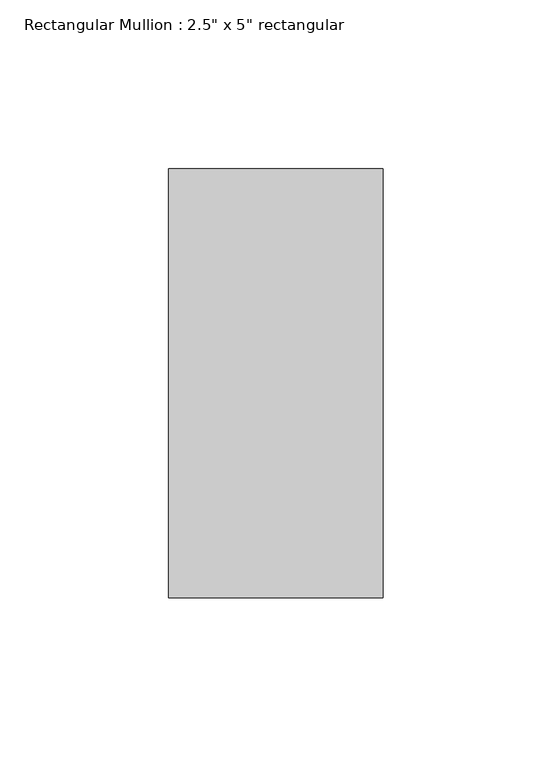
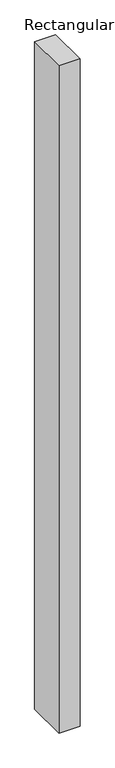
"""IFC4 building model written with IfcOpenShell, lengths in millimetres: member geometry."""

from ifc_helpers import new_model, si_unit, frame, origin, place, context, project, spatial, polyline, outline, extrude, source, transform, mapped, element, save


def member_3374d9b6(model_context):
    return source(origin(), model_context, "Body", "SweptSolid", [
        extrude(outline(polyline([(0.0, 63.5), (0.0, -63.5), (-63.5, -63.5), (-63.5, 63.5), (0.0, 63.5)])), frame((0.0, 0.0, -2133.6), z_axis=(0.0, 0.0, 1.0), x_axis=(1.0, 0.0, 0.0)), (0.0, 0.0, 1.0), 2133.6),
    ])


if __name__ == "__main__":
    model = new_model("IFC4")
    model_context = context("Model", 3, world=origin())
    ifc_project = project(units=[si_unit("LENGTHUNIT", "METRE", prefix="MILLI")], contexts=[model_context])
    site = spatial("IfcSite", under=ifc_project)
    building = spatial("IfcBuilding", under=site)
    placement = place(None, origin())
    member_shape = member_3374d9b6(model_context)
    element("IfcMember", 1, ObjectType="Rectangular Mullion : 2.5\" x 5\" rectangular", at=placement, inside=building, context=model_context, shape_type="MappedRepresentation", body=[
        mapped(member_shape, transform((0.0, 0.0, 0.0), x_axis=(1.0, 0.0, 0.0), y_axis=(0.0, 1.0, 0.0), z_axis=(0.0, 0.0, 1.0))),
    ])
    save(model, "model.ifc")

# Revit data of these elements
# Type "Rectangular Mullion : 2.5\" x 5\" rectangular"
#   built-in parameter 1007304 = 0.416667 (stored number, unit not read)
#   built-in parameter 1007301 = 0.104167 (stored number, unit not read)
#   built-in parameter 1007300 = 0.104167 (stored number, unit not read)
# Element 1 (IfcMember, "Rectangular Mullion : 2.5\" x 5\" rectangular")
#   Materials on its faces: "Aluminum"
# Materials
#   "Aluminum": class "Metal", colour RGB 247 247 247, transparency 0, Description = "Aluminum 6061", Cost = 0
